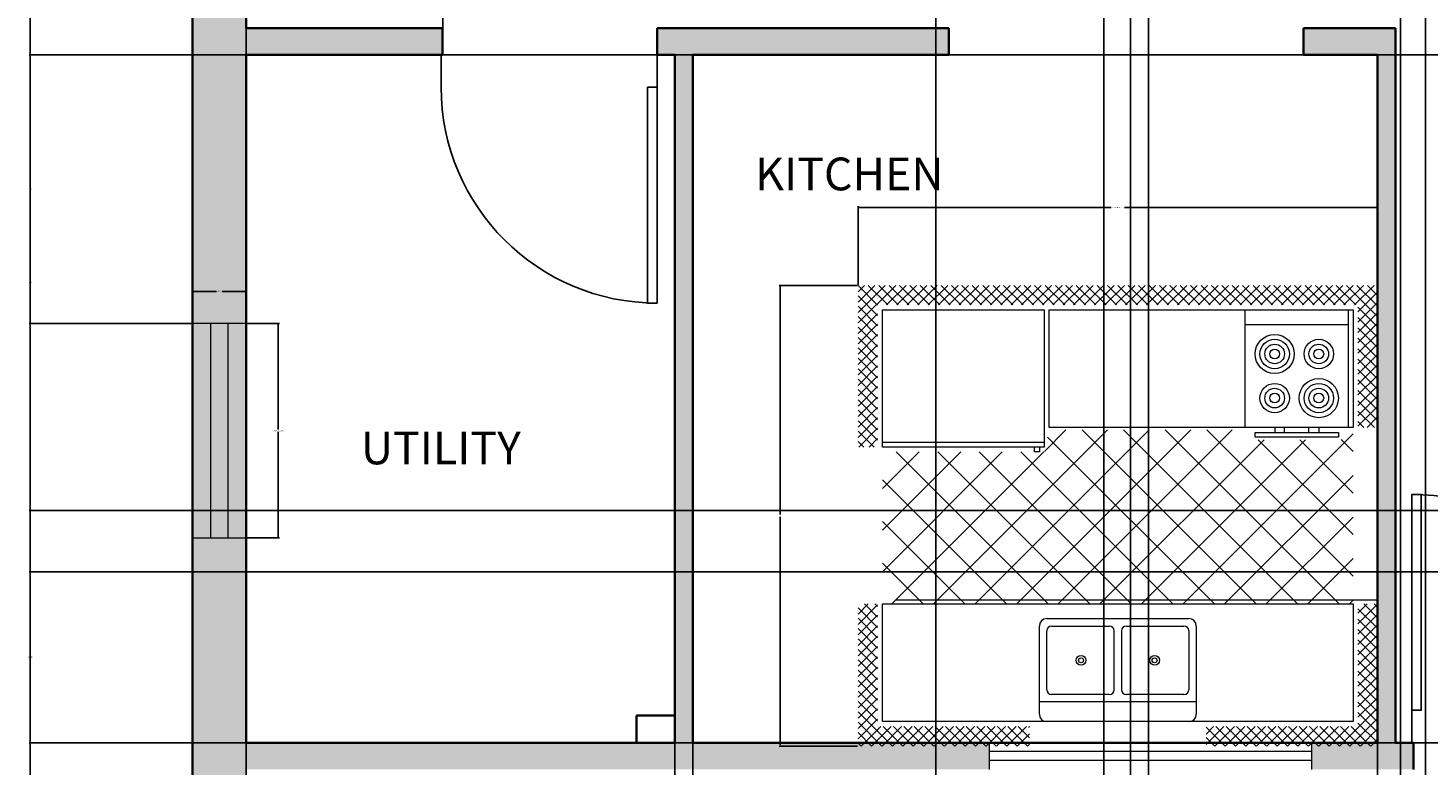
# Model space of a CAD drawing. Units: inches. Extents: x 1839 to 2285, y 722 to 1311.
# Tile 2 of 7: x 1870 to 2105, y 894 to 1018. Entities that reach past the tile are written whole.
import ezdxf

# ---------------------------------------------------------------- set-up
doc = ezdxf.new("R2010")
doc.units = ezdxf.units.IN
for name, color, linetype, lineweight in [('A-ANNO-DIMS', 2, 'Continuous', 18), ('A-AREA-IDEN', 7, 'Continuous', 18), ('A-DOOR', 3, 'Continuous', 25), ('A-FLOR-FIXT', 9, 'Continuous', 18), ('A-GLAZ', 4, 'Continuous', 18), ('A-GLAZ-PATT', 9, 'Continuous', 13), ('A-WALL', 7, 'Continuous', 35)]:
    doc.layers.add(name, color=color, linetype=linetype, lineweight=lineweight)
doc.layers.add('A-WALL-PATT', color=18, linetype='Continuous', lineweight=13, true_color=0x000000)
doc.styles.get("Standard").update_dxf_attribs({"font": 'arial.ttf'})
doc.dimstyles.get("Standard").update_dxf_attribs({"dimtxt": 0.18, "dimasz": 0.18, "dimexe": 0.18, "dimexo": 0.0625, "dimgap": 0.09, "dimtad": 0, "dimtih": 1, "dimtoh": 1, "dimdec": 4, "dimzin": 0, "dimdsep": 46, "dimtxsty": 'Standard', "dimcen": 0.09, "dimadec": 0, "dimazin": 0, "dimtfac": 1, "dimtdec": 4, "dimtofl": 0, "dimtmove": 0, "dimatfit": 3, "dimfxl": 1, "dimtolj": 1, "dimtzin": 0, "dimarcsym": 0})

# ---------------------------------------------------------------- blocks, each defined once
blk = doc.blocks.new('*U4')
for p, q in [((0, 0), (0, -6)), ((40, 0), (40, -6))]:
    blk.add_line(p, q)
blk.add_lwpolyline([(0, 0), (0, 40), (1.75, 40), (1.75, 0)], close=True)
blk.add_arc((0, 0), 40, 0, 90)
blk = doc.blocks.new('*U5')
for p, q in [((0, 0), (0, -6)), ((40, 0), (40, -6))]:
    blk.add_line(p, q)
blk.add_lwpolyline([(0, 0), (0, 40), (1.75, 40), (1.75, 0)], close=True)
blk.add_arc((0, 0), 40, 0, 90)
blk = doc.blocks.new('Kitchen Layout - 7 x 8 ft')
for p, q in [((-5, 81.32), (2.68, 89)), ((-5, 83.44), (0.56, 89)), ((-5, 85.56), (-1.56, 89)), ((-5, 87.68), (-3.68, 89)), ((-1, 84.97), (-5, 88.97)), ((1.09, 85), (-2.91, 89)), ((3.21, 85), (-0.79, 89)), ((0.81, 85), (4.81, 89)), ((5.34, 85), (1.34, 89)), ((2.93, 85), (6.93, 89)), ((7.46, 85), (3.46, 89)), ((5.05, 85), (9.05, 89)), ((9.58, 85), (5.58, 89)), ((7.17, 85), (11.17, 89)), ((11.7, 85), (7.7, 89)), ((9.29, 85), (13.29, 89)), ((13.82, 85), (9.82, 89)), ((11.41, 85), (15.41, 89)), ((15.94, 85), (11.94, 89)), ((13.53, 85), (17.53, 89)), ((18.06, 85), (14.06, 89)), ((15.65, 85), (19.65, 89)), ((20.18, 85), (16.18, 89)), ((17.78, 85), (21.78, 89)), ((22.31, 85), (18.31, 89)), ((19.9, 85), (23.9, 89)), ((24.43, 85), (20.43, 89)), ((22.02, 85), (26.02, 89)), ((26.55, 85), (22.55, 89)), ((24.14, 85), (28.14, 89)), ((28.67, 85), (24.67, 89)), ((26.26, 85), (30.26, 89)), ((30.79, 85), (26.79, 89)), ((28.38, 85), (32.38, 89)), ((32.91, 85), (28.91, 89)), ((30.5, 85), (34.5, 89)), ((35.03, 85), (31.03, 89)), ((32.63, 85), (36.63, 89)), ((37.16, 85), (33.16, 89)), ((34.75, 85), (38.75, 89)), ((39.28, 85), (35.28, 89)), ((36.87, 85), (40.87, 89)), ((41.4, 85), (37.4, 89)), ((38.99, 85), (42.99, 89)), ((43.52, 85), (39.52, 89)), ((41.11, 85), (45.11, 89)), ((45.64, 85), (41.64, 89)), ((43.23, 85), (47.23, 89)), ((47.76, 85), (43.76, 89)), ((45.35, 85), (49.35, 89)), ((49.88, 85), (45.88, 89)), ((47.47, 85), (51.47, 89)), ((52, 85), (48, 89)), ((49.6, 85), (53.6, 89)), ((54.13, 85), (50.13, 89)), ((51.72, 85), (55.72, 89)), ((56.25, 85), (52.25, 89)), ((53.84, 85), (57.84, 89)), ((58.37, 85), (54.37, 89)), ((55.96, 85), (59.96, 89)), ((60.49, 85), (56.49, 89)), ((58.08, 85), (62.08, 89)), ((62.61, 85), (58.61, 89)), ((60.2, 85), (64.2, 89)), ((64.73, 85), (60.73, 89)), ((62.32, 85), (66.32, 89)), ((66.85, 85), (62.85, 89)), ((64.45, 85), (68.45, 89)), ((68.97, 85), (64.97, 89)), ((66.57, 85), (70.57, 89)), ((71.1, 85), (67.1, 89)), ((68.69, 85), (72.69, 89)), ((73.22, 85), (69.22, 89)), ((70.81, 85), (74.81, 89)), ((75.34, 85), (71.34, 89)), ((72.93, 85), (76.93, 89)), ((77.46, 85), (73.46, 89)), ((75.05, 85), (79.05, 89)), ((79.58, 85), (75.58, 89)), ((77.17, 85), (81.17, 89)), ((81.7, 85), (77.7, 89)), ((79.29, 85), (83.29, 89)), ((83.82, 85), (79.82, 89)), ((81.42, 85), (85.42, 89)), ((85.95, 85), (81.95, 89)), ((83.54, 85), (87.54, 89)), ((88.07, 85), (84.07, 89)), ((85.66, 85), (89.66, 89)), ((90.19, 85), (86.19, 89)), ((87.78, 85), (91.78, 89)), ((92.31, 85), (88.31, 89)), ((89.9, 85), (93.9, 89)), ((94.43, 85), (90.43, 89)), ((92.02, 85), (96.02, 89)), ((96.55, 85), (92.55, 89)), ((94.14, 85), (98.14, 89)), ((101, 82.67), (94.67, 89)), ((96.27, 85), (100.27, 89)), ((101, 84.79), (96.79, 89)), ((101, 86.92), (98.92, 89)), ((-1, 82.85), (-5, 86.85)), ((97, 83.61), (101, 87.61)), ((-1, 80.73), (-5, 84.73)), ((-5, 79.19), (-1, 83.19)), ((34, 84), (96, 84)), ((34, 60), (34, 84)), ((96, 84), (96, 60)), ((97, 81.49), (101, 85.49)), ((101, 80.55), (97, 84.55)), ((97, 79.37), (101, 83.37)), ((-1, 78.61), (-5, 82.61)), ((-5, 77.07), (-1, 81.07)), ((-1, 76.49), (-5, 80.49)), ((74, 81), (95, 81)), ((101, 78.43), (97, 82.43)), ((97, 77.25), (101, 81.25)), ((101, 76.31), (97, 80.31)), ((-5, 74.95), (-1, 78.95)), ((-1, 74.36), (-5, 78.36)), ((97, 75.13), (101, 79.13)), ((101, 74.19), (97, 78.19)), ((-5, 72.83), (-1, 76.83)), ((-1, 72.24), (-5, 76.24)), ((-5, 70.71), (-1, 74.71)), ((97, 73.01), (101, 77.01)), ((101, 72.07), (97, 76.07)), ((97, 70.89), (101, 74.89)), ((-1, 70.12), (-5, 74.12)), ((-5, 68.59), (-1, 72.59)), ((-1, 68), (-5, 72)), ((101, 69.95), (97, 73.95)), ((97, 68.76), (101, 72.76)), ((101, 67.82), (97, 71.82)), ((-5, 66.47), (-1, 70.47)), ((-1, 65.88), (-5, 69.88)), ((97, 66.64), (101, 70.64)), ((101, 65.7), (97, 69.7)), ((-5, 64.35), (-1, 68.35)), ((-1, 63.76), (-5, 67.76)), ((-5, 62.22), (-1, 66.22)), ((97, 64.52), (101, 68.52)), ((101, 63.58), (97, 67.58)), ((97, 62.4), (101, 66.4)), ((-1, 61.64), (-5, 65.64)), ((-5, 60.1), (-1, 64.1)), ((-1, 59.52), (-5, 63.52)), ((101, 61.46), (97, 65.46)), ((97, 60.28), (101, 64.28)), ((100.34, 60), (97, 63.34)), ((-5, 57.98), (-1, 61.98)), ((-1, 57.39), (-5, 61.39)), ((96, 60), (34, 60)), ((80, 60), (80, 59)), ((82, 59), (82, 60)), ((87, 59), (87, 60)), ((89, 60), (89, 59)), ((98.22, 60), (97, 61.22)), ((98.84, 60), (101, 62.16)), ((100.96, 60), (101, 60.04)), ((-1.73, 56), (-5, 59.27)), ((-3.85, 56), (-5, 57.15)), ((-4.86, 56), (-1, 59.86)), ((-2.74, 56), (-1, 57.74)), ((10.4, 24), (45.9, 59.5)), ((18.88, 24), (54.38, 59.5)), ((27.37, 24), (62.87, 59.5)), ((33.03, 55.11), (37.41, 59.5)), ((67.71, 24), (33.68, 58.04)), ((35.85, 24), (71.35, 59.5)), ((76.2, 24), (40.7, 59.5)), ((44.34, 24), (77.84, 57.5)), ((84.68, 24), (49.18, 59.5)), ((52.82, 24), (86.32, 57.5)), ((93.17, 24), (57.67, 59.5)), ((61.31, 24), (96, 58.69)), ((96, 29.65), (66.15, 59.5)), ((96, 38.14), (76.64, 57.5)), ((96, 46.63), (85.13, 57.5)), ((96, 55.11), (93.57, 57.54)), ((0, 57), (33, 57)), ((0, 30.57), (24.43, 55)), ((0, 39.06), (15.94, 55)), ((0, 47.54), (7.46, 55)), ((1.91, 24), (32.91, 55)), ((33.77, 24), (2.77, 55)), ((42.26, 24), (11.26, 55)), ((50.74, 24), (19.74, 55)), ((59.23, 24), (28.23, 55)), ((31, 55), (31, 56)), ((32, 55), (31, 55)), ((32, 56), (32, 55)), ((25.29, 24), (0, 49.29)), ((69.79, 24), (96, 50.21)), ((16.8, 24), (0, 40.8)), ((78.28, 24), (96, 41.72)), ((8.32, 24), (0, 32.32)), ((86.76, 24), (96, 33.24)), ((-5, 21.92), (-2.92, 24)), ((-5, 19.8), (-1, 23.8)), ((-1, 19.21), (-5, 23.21)), ((-1, 21.33), (-3.67, 24)), ((-1, 23.45), (-1.55, 24)), ((0, 24), (96, 24)), ((0, 0), (0, 24)), ((95.25, 24), (96, 24.75)), ((96, 24), (96, 0)), ((97, 22.1), (98.9, 24)), ((97, 19.97), (101, 23.97)), ((101, 19.03), (97, 23.03)), ((101, 21.16), (98.16, 24)), ((101, 23.28), (100.28, 24)), ((-5, 17.68), (-1, 21.68)), ((-1, 17.09), (-5, 21.09)), ((97, 17.85), (101, 21.85)), ((101, 16.91), (97, 20.91)), ((-5, 15.55), (-1, 19.55)), ((-1, 14.97), (-5, 18.97)), ((-5, 13.43), (-1, 17.43)), ((47.25, 6.5), (47.25, 18.5)), ((48.75, 18.5), (48.75, 6.5)), ((97, 15.73), (101, 19.73)), ((101, 14.79), (97, 18.79)), ((97, 13.61), (101, 17.61)), ((-1, 12.85), (-5, 16.85)), ((-5, 11.31), (-1, 15.31)), ((-1, 10.73), (-5, 14.73)), ((101, 12.67), (97, 16.67)), ((97, 11.49), (101, 15.49)), ((101, 10.55), (97, 14.55)), ((-5, 9.19), (-1, 13.19)), ((-1, 8.6), (-5, 12.6)), ((97, 9.37), (101, 13.37)), ((101, 8.43), (97, 12.43)), ((-5, 7.07), (-1, 11.07)), ((-1, 6.48), (-5, 10.48)), ((-5, 4.95), (-1, 8.95)), ((97, 7.25), (101, 11.25)), ((101, 6.31), (97, 10.31)), ((97, 5.12), (101, 9.12)), ((-1, 4.36), (-5, 8.36)), ((-5, 2.83), (-1, 6.83)), ((-1, 2.24), (-5, 6.24)), ((101, 4.18), (97, 8.18)), ((97, 3), (101, 7)), ((101, 2.06), (97, 6.06)), ((-5, 0.71), (-1, 4.71)), ((-1, 0.12), (-5, 4.12)), ((64, 4), (32, 4)), ((97, 0.88), (101, 4.88)), ((101, -0.06), (97, 3.94)), ((-5, -1.42), (-1, 2.58)), ((2, -5), (-5, 2)), ((-5, -3.54), (-1, 0.46)), ((96, 0), (0, 0)), ((93.24, -5), (101, 2.76)), ((95.36, -5), (101, 0.64)), ((101, -2.18), (97, 1.82)), ((-0.12, -5), (-5, -0.12)), ((-2.25, -5), (-5, -2.25)), ((-4.34, -5), (-0.34, -1)), ((-2.22, -5), (1.78, -1)), ((-0.1, -5), (3.9, -1)), ((4.12, -5), (0.12, -1)), ((2.02, -5), (6.02, -1)), ((6.24, -5), (2.24, -1)), ((4.14, -5), (8.14, -1)), ((8.36, -5), (4.36, -1)), ((6.27, -5), (10.27, -1)), ((10.48, -5), (6.48, -1)), ((8.39, -5), (12.39, -1)), ((12.6, -5), (8.6, -1)), ((10.51, -5), (14.51, -1)), ((14.73, -5), (10.73, -1)), ((12.63, -5), (16.63, -1)), ((16.85, -5), (12.85, -1)), ((14.75, -5), (18.75, -1)), ((18.97, -5), (14.97, -1)), ((16.87, -5), (20.87, -1)), ((21.09, -5), (17.09, -1)), ((18.99, -5), (22.99, -1)), ((23.21, -5), (19.21, -1)), ((21.11, -5), (25.11, -1)), ((25.33, -5), (21.33, -1)), ((23.24, -5), (27.24, -1)), ((27.45, -5), (23.45, -1)), ((25.36, -5), (29.36, -1)), ((29.57, -5), (25.57, -1)), ((27.48, -5), (30, -2.48)), ((30, -3.3), (27.7, -1)), ((30, -1.18), (29.82, -1)), ((66, -2.54), (67.54, -1)), ((66, -4.66), (69.66, -1)), ((69.88, -5), (66, -1.12)), ((67.78, -5), (71.78, -1)), ((72, -5), (68, -1)), ((69.9, -5), (73.9, -1)), ((74.12, -5), (70.12, -1)), ((72.03, -5), (76.03, -1)), ((76.24, -5), (72.24, -1)), ((74.15, -5), (78.15, -1)), ((78.36, -5), (74.36, -1)), ((76.27, -5), (80.27, -1)), ((80.49, -5), (76.49, -1)), ((78.39, -5), (82.39, -1)), ((82.61, -5), (78.61, -1)), ((80.51, -5), (84.51, -1)), ((84.73, -5), (80.73, -1)), ((82.63, -5), (86.63, -1)), ((86.85, -5), (82.85, -1)), ((84.75, -5), (88.75, -1)), ((88.97, -5), (84.97, -1)), ((86.88, -5), (90.88, -1)), ((91.09, -5), (87.09, -1)), ((89, -5), (93, -1)), ((93.21, -5), (89.21, -1)), ((91.12, -5), (95.12, -1)), ((95.34, -5), (91.34, -1)), ((97.46, -5), (93.46, -1)), ((99.58, -5), (95.58, -1)), ((101, -4.3), (97, -0.3)), ((97.48, -5), (101, -1.48)), ((-4.37, -5), (-5, -4.37)), ((29.6, -5), (30, -4.6)), ((67.76, -5), (66, -3.24)), ((99.6, -5), (101, -3.6))]:
    blk.add_line(p, q)
for points in [[(0, 56), (0, 84), (33, 84), (33, 56)], [(74, 60), (74, 84), (95, 84), (95, 60)], [(76, 58), (76, 59), (93, 59), (93, 58)]]:
    blk.add_lwpolyline(points, close=True)
for points in [[(33.5, 21), (62.5, 21)], [(32, 1.5), (32, 19.5)], [(33.5, 6.5), (33.5, 18.5)], [(34.5, 19.5), (46.25, 19.5)], [(49.75, 19.5), (61.5, 19.5)], [(62.5, 18.5), (62.5, 6.5)], [(64, 19.5), (64, 1.5)], [(46.25, 5.5), (34.5, 5.5)], [(61.5, 5.5), (49.75, 5.5)], [(62.5, 0), (33.5, 0)]]:
    blk.add_lwpolyline(points)
for centre, radius in [((80, 75), 4), ((80, 75), 3), ((89, 75), 3), ((80, 75), 2), ((80, 75), 1), ((89, 75), 2), ((89, 75), 1), ((80, 66), 3), ((89, 66), 4), ((89, 66), 3), ((80, 66), 2), ((80, 66), 1), ((89, 66), 2), ((89, 66), 1), ((40.5, 12.5), 1), ((40.5, 12.5), 0.5), ((55.5, 12.5), 1), ((55.5, 12.5), 0.5)]:
    blk.add_circle(centre, radius)
for centre, radius, start, end in [((33.5, 19.5), 1.5, 90, 180), ((62.5, 19.5), 1.5, 0, 90), ((34.5, 18.5), 1, 90, 180), ((46.25, 18.5), 1, 0, 90), ((49.75, 18.5), 1, 90, 180), ((61.5, 18.5), 1, 0, 90), ((34.5, 6.5), 1, 180, 270), ((46.25, 6.5), 1, 270, 0), ((49.75, 6.5), 1, 180, 270), ((61.5, 6.5), 1, 270, 0), ((33.5, 1.5), 1.5, 180, 270), ((62.5, 1.5), 1.5, 270, 0)]:
    blk.add_arc(centre, radius, start, end)
blk = doc.blocks.new('WIN-36x9')
for p, q in [((0, 9), (0, 0)), ((36, 9), (0, 9)), ((36, 0), (36, 9)), ((36, 6), (0, 6)), ((0, 3), (36, 3)), ((0, 0), (36, 0))]:
    blk.add_line(p, q)
blk = doc.blocks.new('*D19')
at = {"layer": 'A-ANNO-DIMS', "color": 0, "lineweight": -2, "transparency": 16777216}
for p, q in [((1906.74, 968.21), (1912.26, 968.21)), ((1912.08, 968.03), (1912.08, 950.39)), ((1912.08, 932.39), (1912.08, 950.03)), ((1906.74, 932.21), (1912.26, 932.21))]:
    blk.add_line(p, q, dxfattribs=at)
at = {"layer": 'A-ANNO-DIMS', "color": 0, "transparency": 16777216}
for points in [[(1912.05, 968.03), (1912.11, 968.03), (1912.08, 968.21)], [(1912.05, 932.39), (1912.11, 932.39), (1912.08, 932.21)]]:
    blk.add_solid(points, dxfattribs=at)
at = {"layer": 'Defpoints', "color": 0, "transparency": 16777216}
for p in [(1906.68, 968.21), (1906.68, 932.21), (1912.08, 932.21)]:
    blk.add_point(p, dxfattribs=at)
at = {"layer": 'A-ANNO-DIMS', "color": 0, "transparency": 16777216, "insert": (1912.08, 950.21), "char_height": 0.18, "attachment_point": 5}
blk.add_mtext('\\A1;WINDOW 36 TYP.', dxfattribs=at)
blk = doc.blocks.new('*D20')
at = {"layer": 'A-ANNO-DIMS', "color": 0, "lineweight": -2, "transparency": 16777216}
for p, q in [((1897.68, 968.27), (1897.68, 973.79)), ((1897.86, 973.61), (1901.72, 973.61)), ((1906.5, 973.61), (1902.64, 973.61)), ((1906.68, 968.27), (1906.68, 973.79))]:
    blk.add_line(p, q, dxfattribs=at)
at = {"layer": 'A-ANNO-DIMS', "color": 0, "transparency": 16777216}
for points in [[(1897.86, 973.64), (1897.86, 973.58), (1897.68, 973.61)], [(1906.5, 973.64), (1906.5, 973.58), (1906.68, 973.61)]]:
    blk.add_solid(points, dxfattribs=at)
at = {"layer": 'Defpoints', "color": 0, "transparency": 16777216}
for p in [(1906.68, 973.61), (1897.68, 968.21), (1906.68, 968.21)]:
    blk.add_point(p, dxfattribs=at)
at = {"layer": 'A-ANNO-DIMS', "color": 0, "transparency": 16777216, "insert": (1902.18, 973.61), "char_height": 0.18, "attachment_point": 5}
blk.add_mtext('\\A1;9 TYP.', dxfattribs=at)
blk = doc.blocks.new('*D35')
at = {"layer": 'A-ANNO-DIMS', "color": 0, "lineweight": -2, "transparency": 16777216}
for p, q in [((2009.42, 974.68), (2009.42, 987.89)), ((2009.6, 987.71), (2051.91, 987.71)), ((2096.48, 987.71), (2054.17, 987.71)), ((2096.66, 974.68), (2096.66, 987.89))]:
    blk.add_line(p, q, dxfattribs=at)
at = {"layer": 'A-ANNO-DIMS', "color": 0, "transparency": 16777216}
for points in [[(2009.6, 987.74), (2009.6, 987.68), (2009.42, 987.71)], [(2096.48, 987.74), (2096.48, 987.68), (2096.66, 987.71)]]:
    blk.add_solid(points, dxfattribs=at)
at = {"layer": 'Defpoints', "color": 0, "transparency": 16777216}
for p in [(2096.66, 987.71), (2009.42, 974.62), (2096.66, 974.62)]:
    blk.add_point(p, dxfattribs=at)
at = {"layer": 'A-ANNO-DIMS', "color": 0, "transparency": 16777216, "insert": (2053.04, 987.71), "char_height": 0.18, "attachment_point": 5}
blk.add_mtext('\\A1;KITCHEN UNIT 87', dxfattribs=at)
blk = doc.blocks.new('*D36')
at = {"layer": 'A-ANNO-DIMS', "color": 0, "lineweight": -2, "transparency": 16777216}
for p, q in [((2009.36, 974.62), (1996.16, 974.62)), ((1996.34, 974.44), (1996.34, 936.12)), ((1996.34, 897.44), (1996.34, 935.76)), ((2009.36, 897.26), (1996.16, 897.26))]:
    blk.add_line(p, q, dxfattribs=at)
at = {"layer": 'A-ANNO-DIMS', "color": 0, "transparency": 16777216}
for points in [[(1996.31, 974.44), (1996.37, 974.44), (1996.34, 974.62)], [(1996.31, 897.44), (1996.37, 897.44), (1996.34, 897.26)]]:
    blk.add_solid(points, dxfattribs=at)
at = {"layer": 'Defpoints', "color": 0, "transparency": 16777216}
for p in [(1996.34, 974.62), (2009.42, 974.62), (2009.42, 897.26)]:
    blk.add_point(p, dxfattribs=at)
at = {"layer": 'A-ANNO-DIMS', "color": 0, "transparency": 16777216, "insert": (1996.34, 935.94), "char_height": 0.18, "attachment_point": 5}
blk.add_mtext('\\A1;77', dxfattribs=at)
blk = doc.blocks.new('*D42')
at = {"layer": 'A-ANNO-DIMS', "color": 0, "lineweight": -2, "transparency": 16777216}
for p, q in [((1897.61, 1283.33), (1870.25, 1283.33)), ((1870.43, 1283.15), (1870.43, 1043.51)), ((1870.43, 803.51), (1870.43, 1043.15)), ((1897.61, 803.33), (1870.25, 803.33))]:
    blk.add_line(p, q, dxfattribs=at)
at = {"layer": 'A-ANNO-DIMS', "color": 0, "transparency": 16777216}
for points in [[(1870.4, 1283.15), (1870.46, 1283.15), (1870.43, 1283.33)], [(1870.4, 803.51), (1870.46, 803.51), (1870.43, 803.33)]]:
    blk.add_solid(points, dxfattribs=at)
at = {"layer": 'Defpoints', "color": 0, "transparency": 16777216}
for p in [(1870.43, 1283.33), (1897.68, 1283.33), (1897.68, 803.33)]:
    blk.add_point(p, dxfattribs=at)
at = {"layer": 'A-ANNO-DIMS', "color": 0, "transparency": 16777216, "insert": (1870.43, 1043.33), "char_height": 0.18, "attachment_point": 5}
blk.add_mtext('\\A1;480', dxfattribs=at)
blk = doc.blocks.new('*D43')
at = {"layer": 'A-ANNO-DIMS', "color": 0, "lineweight": -2, "transparency": 16777216}
for p, q in [((2050.68, 1145.27), (2050.68, 722.34)), ((1906.68, 1142.27), (1906.68, 722.34)), ((1906.86, 722.52), (1978.4, 722.52)), ((2050.5, 722.52), (1978.96, 722.52))]:
    blk.add_line(p, q, dxfattribs=at)
at = {"layer": 'A-ANNO-DIMS', "color": 0, "transparency": 16777216}
for points in [[(1906.86, 722.55), (1906.86, 722.49), (1906.68, 722.52)], [(2050.5, 722.55), (2050.5, 722.49), (2050.68, 722.52)]]:
    blk.add_solid(points, dxfattribs=at)
at = {"layer": 'Defpoints', "color": 0, "transparency": 16777216}
for p in [(2050.68, 1145.33), (1906.68, 1142.33), (2050.68, 722.52)]:
    blk.add_point(p, dxfattribs=at)
at = {"layer": 'A-ANNO-DIMS', "color": 0, "transparency": 16777216, "insert": (1978.68, 722.52), "char_height": 0.18, "attachment_point": 5}
blk.add_mtext('\\A1;144', dxfattribs=at)
blk = doc.blocks.new('*D44')
at = {"layer": 'A-ANNO-DIMS', "color": 0, "lineweight": -2, "transparency": 16777216}
for p, q in [((2055.18, 1137.77), (2055.18, 722.34)), ((2104.68, 1137.77), (2104.68, 722.34)), ((2055.36, 722.52), (2079.6, 722.52)), ((2104.5, 722.52), (2080.26, 722.52))]:
    blk.add_line(p, q, dxfattribs=at)
at = {"layer": 'A-ANNO-DIMS', "color": 0, "transparency": 16777216}
for points in [[(2055.36, 722.55), (2055.36, 722.49), (2055.18, 722.52)], [(2104.5, 722.55), (2104.5, 722.49), (2104.68, 722.52)]]:
    blk.add_solid(points, dxfattribs=at)
at = {"layer": 'Defpoints', "color": 0, "transparency": 16777216}
for p in [(2055.18, 1137.83), (2104.68, 1137.83), (2104.68, 722.52)]:
    blk.add_point(p, dxfattribs=at)
at = {"layer": 'A-ANNO-DIMS', "color": 0, "transparency": 16777216, "insert": (2079.93, 722.52), "char_height": 0.18, "attachment_point": 5}
blk.add_mtext('\\A1;49.5', dxfattribs=at)
blk = doc.blocks.new('*D51')
at = {"layer": 'A-ANNO-DIMS', "color": 0, "lineweight": -2, "transparency": 16777216}
for p, q in [((1906.68, 897.77), (1906.68, 722.34)), ((1978.68, 897.77), (1978.68, 722.34)), ((1906.86, 722.52), (1942.46, 722.52)), ((1978.5, 722.52), (1942.89, 722.52))]:
    blk.add_line(p, q, dxfattribs=at)
at = {"layer": 'A-ANNO-DIMS', "color": 0, "transparency": 16777216}
for points in [[(1906.86, 722.55), (1906.86, 722.49), (1906.68, 722.52)], [(1978.5, 722.55), (1978.5, 722.49), (1978.68, 722.52)]]:
    blk.add_solid(points, dxfattribs=at)
at = {"layer": 'Defpoints', "color": 0, "transparency": 16777216}
for p in [(1906.68, 897.83), (1978.68, 897.83), (1978.68, 722.52)]:
    blk.add_point(p, dxfattribs=at)
at = {"layer": 'A-ANNO-DIMS', "color": 0, "transparency": 16777216, "insert": (1942.68, 722.52), "char_height": 0.18, "attachment_point": 5}
blk.add_mtext('\\A1;72', dxfattribs=at)
blk = doc.blocks.new('*D52')
at = {"layer": 'A-ANNO-DIMS', "color": 0, "lineweight": -2, "transparency": 16777216}
for p, q in [((1981.68, 1013.27), (1981.68, 722.34)), ((2096.66, 1013.27), (2096.66, 722.34)), ((1981.86, 722.52), (2038.72, 722.52)), ((2096.48, 722.52), (2039.63, 722.52))]:
    blk.add_line(p, q, dxfattribs=at)
at = {"layer": 'A-ANNO-DIMS', "color": 0, "transparency": 16777216}
for points in [[(1981.86, 722.55), (1981.86, 722.49), (1981.68, 722.52)], [(2096.48, 722.55), (2096.48, 722.49), (2096.66, 722.52)]]:
    blk.add_solid(points, dxfattribs=at)
at = {"layer": 'Defpoints', "color": 0, "transparency": 16777216}
for p in [(1981.68, 1013.33), (2096.66, 1013.33), (2096.66, 722.52)]:
    blk.add_point(p, dxfattribs=at)
at = {"layer": 'A-ANNO-DIMS', "color": 0, "transparency": 16777216, "insert": (2039.17, 722.52), "char_height": 0.18, "attachment_point": 5}
blk.add_mtext('\\A1;114.99', dxfattribs=at)
blk = doc.blocks.new('*D55')
at = {"layer": 'A-ANNO-DIMS', "color": 0, "lineweight": -2, "transparency": 16777216}
for p, q in [((2022.5, 812.39), (2022.5, 1310.76)), ((2022.68, 1310.58), (2061.29, 1310.58)), ((2100.32, 1310.58), (2061.72, 1310.58)), ((2100.5, 812.39), (2100.5, 1310.76))]:
    blk.add_line(p, q, dxfattribs=at)
at = {"layer": 'A-ANNO-DIMS', "color": 0, "transparency": 16777216}
for points in [[(2022.68, 1310.61), (2022.68, 1310.55), (2022.5, 1310.58)], [(2100.32, 1310.61), (2100.32, 1310.55), (2100.5, 1310.58)]]:
    blk.add_solid(points, dxfattribs=at)
at = {"layer": 'Defpoints', "color": 0, "transparency": 16777216}
for p in [(2100.5, 1310.58), (2022.5, 812.33), (2100.5, 812.33)]:
    blk.add_point(p, dxfattribs=at)
at = {"layer": 'A-ANNO-DIMS', "color": 0, "transparency": 16777216, "insert": (2061.5, 1310.58), "char_height": 0.18, "attachment_point": 5}
blk.add_mtext('\\A1;78', dxfattribs=at)
blk = doc.blocks.new('*D63')
at = {"layer": 'A-ANNO-DIMS', "color": 0, "lineweight": -2, "transparency": 16777216}
for p, q in [((1906.61, 1013.33), (1870.25, 1013.33)), ((1870.43, 1013.15), (1870.43, 990.95)), ((1870.43, 968.39), (1870.43, 990.59)), ((1897.61, 968.21), (1870.25, 968.21))]:
    blk.add_line(p, q, dxfattribs=at)
at = {"layer": 'A-ANNO-DIMS', "color": 0, "transparency": 16777216}
for points in [[(1870.4, 1013.15), (1870.46, 1013.15), (1870.43, 1013.33)], [(1870.4, 968.39), (1870.46, 968.39), (1870.43, 968.21)]]:
    blk.add_solid(points, dxfattribs=at)
at = {"layer": 'Defpoints', "color": 0, "transparency": 16777216}
for p in [(1870.43, 1013.33), (1906.68, 1013.33), (1897.68, 968.21)]:
    blk.add_point(p, dxfattribs=at)
at = {"layer": 'A-ANNO-DIMS', "color": 0, "transparency": 16777216, "insert": (1870.43, 990.77), "char_height": 0.18, "attachment_point": 5}
blk.add_mtext('\\A1;45.12', dxfattribs=at)
blk = doc.blocks.new('*D64')
at = {"layer": 'A-ANNO-DIMS', "color": 0, "lineweight": -2, "transparency": 16777216}
for p, q in [((2248.61, 926.49), (1870.25, 926.49)), ((1870.43, 926.31), (1870.43, 912.34)), ((1870.43, 898.01), (1870.43, 911.98)), ((2248.61, 897.83), (1870.25, 897.83))]:
    blk.add_line(p, q, dxfattribs=at)
at = {"layer": 'A-ANNO-DIMS', "color": 0, "transparency": 16777216}
for points in [[(1870.4, 926.31), (1870.46, 926.31), (1870.43, 926.49)], [(1870.4, 898.01), (1870.46, 898.01), (1870.43, 897.83)]]:
    blk.add_solid(points, dxfattribs=at)
at = {"layer": 'Defpoints', "color": 0, "transparency": 16777216}
for p in [(1870.43, 926.49), (2248.68, 926.49), (2248.68, 897.83)]:
    blk.add_point(p, dxfattribs=at)
at = {"layer": 'A-ANNO-DIMS', "color": 0, "transparency": 16777216, "insert": (1870.43, 912.16), "char_height": 0.18, "attachment_point": 5}
blk.add_mtext('\\A1;28.655', dxfattribs=at)
blk = doc.blocks.new('*D71')
at = {"layer": 'A-ANNO-DIMS', "color": 0, "lineweight": -2, "transparency": 16777216}
for p, q in [((1978.68, 897.77), (1978.68, 722.34)), ((1981.68, 897.77), (1981.68, 722.34)), ((1978.86, 722.52), (1980.03, 722.52)), ((1981.5, 722.52), (1980.33, 722.52))]:
    blk.add_line(p, q, dxfattribs=at)
at = {"layer": 'A-ANNO-DIMS', "color": 0, "transparency": 16777216}
for points in [[(1978.86, 722.55), (1978.86, 722.49), (1978.68, 722.52)], [(1981.5, 722.55), (1981.5, 722.49), (1981.68, 722.52)]]:
    blk.add_solid(points, dxfattribs=at)
at = {"layer": 'Defpoints', "color": 0, "transparency": 16777216}
for p in [(1978.68, 897.83), (1981.68, 897.83), (1981.68, 722.52)]:
    blk.add_point(p, dxfattribs=at)
at = {"layer": 'A-ANNO-DIMS', "color": 0, "transparency": 16777216, "insert": (1980.18, 722.52), "char_height": 0.18, "attachment_point": 5}
blk.add_mtext('\\A1;3', dxfattribs=at)
blk = doc.blocks.new('*D81')
at = {"layer": 'A-ANNO-DIMS', "color": 0, "lineweight": -2, "transparency": 16777216}
for p, q in [((1906.68, 1013.39), (1906.68, 1310.76)), ((1906.86, 1310.58), (1922.96, 1310.58)), ((1939.5, 1310.58), (1923.4, 1310.58)), ((1939.68, 1013.39), (1939.68, 1310.76))]:
    blk.add_line(p, q, dxfattribs=at)
at = {"layer": 'A-ANNO-DIMS', "color": 0, "transparency": 16777216}
for points in [[(1906.86, 1310.61), (1906.86, 1310.55), (1906.68, 1310.58)], [(1939.5, 1310.61), (1939.5, 1310.55), (1939.68, 1310.58)]]:
    blk.add_solid(points, dxfattribs=at)
at = {"layer": 'Defpoints', "color": 0, "transparency": 16777216}
for p in [(1939.68, 1310.58), (1906.68, 1013.33), (1939.68, 1013.33)]:
    blk.add_point(p, dxfattribs=at)
at = {"layer": 'A-ANNO-DIMS', "color": 0, "transparency": 16777216, "insert": (1923.18, 1310.58), "char_height": 0.18, "attachment_point": 5}
blk.add_mtext('\\A1;33', dxfattribs=at)
blk = doc.blocks.new('*D82')
at = {"layer": 'A-ANNO-DIMS', "color": 0, "lineweight": -2, "transparency": 16777216}
for p, q in [((2164.61, 1013.33), (1870.25, 1013.33)), ((1870.43, 1013.15), (1870.43, 975.26)), ((1870.43, 937.01), (1870.43, 974.9)), ((2164.61, 936.83), (1870.25, 936.83))]:
    blk.add_line(p, q, dxfattribs=at)
at = {"layer": 'A-ANNO-DIMS', "color": 0, "transparency": 16777216}
for points in [[(1870.4, 1013.15), (1870.46, 1013.15), (1870.43, 1013.33)], [(1870.4, 937.01), (1870.46, 937.01), (1870.43, 936.83)]]:
    blk.add_solid(points, dxfattribs=at)
at = {"layer": 'Defpoints', "color": 0, "transparency": 16777216}
for p in [(1870.43, 1013.33), (2164.68, 1013.33), (2164.68, 936.83)]:
    blk.add_point(p, dxfattribs=at)
at = {"layer": 'A-ANNO-DIMS', "color": 0, "transparency": 16777216, "insert": (1870.43, 975.08), "char_height": 0.18, "attachment_point": 5}
blk.add_mtext('\\A1;76.5', dxfattribs=at)
blk = doc.blocks.new('*D84')
at = {"layer": 'A-ANNO-DIMS', "color": 0, "lineweight": -2, "transparency": 16777216}
for p, q in [((2055.18, 1218.77), (2055.18, 722.34)), ((2058.18, 1218.77), (2058.18, 722.34)), ((2055.36, 722.52), (2056.53, 722.52)), ((2058, 722.52), (2056.83, 722.52))]:
    blk.add_line(p, q, dxfattribs=at)
at = {"layer": 'A-ANNO-DIMS', "color": 0, "transparency": 16777216}
for points in [[(2055.36, 722.55), (2055.36, 722.49), (2055.18, 722.52)], [(2058, 722.55), (2058, 722.49), (2058.18, 722.52)]]:
    blk.add_solid(points, dxfattribs=at)
at = {"layer": 'Defpoints', "color": 0, "transparency": 16777216}
for p in [(2055.18, 1218.83), (2058.18, 1218.83), (2058.18, 722.52)]:
    blk.add_point(p, dxfattribs=at)
at = {"layer": 'A-ANNO-DIMS', "color": 0, "transparency": 16777216, "insert": (2056.68, 722.52), "char_height": 0.18, "attachment_point": 5}
blk.add_mtext('\\A1;3', dxfattribs=at)

msp = doc.modelspace()

# ---------------------------------------------------------------- hatches: boundary and pattern name
at = {"layer": 'A-GLAZ-PATT'}
h = msp.add_hatch(color=256, dxfattribs=at)
h.dxf.hatch_style = 1
h.set_gradient(color1=(0, 0, 255), color2=(255, 255, 0), name='INVCYLINDER')
h.paths.add_polyline_path([(1900.6771, 968.2107), (1897.6771, 968.2107), (1897.6771, 932.2107), (1900.6771, 932.2107)])
h.paths.add_polyline_path([(1903.6771, 968.2107), (1900.6771, 968.2107), (1900.6771, 932.2107), (1903.6771, 932.2107)])
h.paths.add_polyline_path([(1906.6771, 968.2107), (1903.6771, 968.2107), (1903.6771, 932.2107), (1906.6771, 932.2107)])
at = {"layer": 'A-WALL-PATT'}
h = msp.add_hatch(color=256, dxfattribs=at)
h.dxf.hatch_style = 1
h.paths.add_polyline_path([(1906.6771, 1274.3314), (1942.6771, 1274.3314), (1942.6771, 1283.3314), (1897.6771, 1283.3314), (1897.6771, 968.2107), (1906.6771, 968.2107), (1906.6771, 1013.3314), (1939.6771, 1013.3314), (1939.6771, 1017.8314), (1906.6771, 1017.8314), (1906.6771, 1137.8314), (2050.6771, 1137.8314), (2050.6771, 1142.3314), (1906.6771, 1142.3314)])
h.paths.add_polyline_path([(2064.0508, 1283.3314), (1978.6771, 1283.3314), (1978.6771, 1274.3314), (2050.6771, 1274.3314), (2050.6771, 1184.3314), (2055.1771, 1184.3314), (2055.1771, 1214.3314), (2058.1771, 1214.3314), (2058.1771, 1218.8314), (2055.1771, 1218.8314), (2055.1771, 1274.3314), (2064.0508, 1274.3314)])
h.paths.add_polyline_path([(2182.6416, 1283.3314), (2088.0508, 1283.3314), (2088.0508, 1274.3314), (2104.6771, 1274.3314), (2104.6771, 1218.8314), (2094.1771, 1218.8314), (2094.1771, 1214.3314), (2104.6771, 1214.3314), (2104.6771, 1184.3314), (2109.1771, 1184.3314), (2109.1771, 1274.3314), (2182.6416, 1274.3314)])
h.paths.add_polyline_path([(2257.6771, 1283.3314), (2218.6416, 1283.3314), (2218.6416, 1274.3314), (2248.6771, 1274.3314), (2248.6771, 1142.3314), (2186.4004, 1142.3314), (2109.1771, 1142.3314), (2109.1771, 1137.8314), (2248.6771, 1137.8314), (2248.6771, 1094.9086), (2257.6771, 1094.9086)])
h.paths.add_polyline_path([(2257.6771, 1058.9086), (2248.6771, 1058.9086), (2248.6771, 1017.8314), (2160.1771, 1017.8314), (2160.1771, 939.8314), (2164.6771, 939.8314), (2164.6771, 1013.3314), (2248.6771, 1013.3314), (2248.6771, 977.3314), (2248.6771, 950.4862), (2257.6771, 950.4862)])
h.paths.add_polyline_path([(2257.6771, 893.3314), (2248.6771, 893.3314), (2248.6771, 850.1143), (2190.4862, 850.1143), (2190.4862, 845.6143), (2248.6771, 845.6143), (2248.6771, 812.3314), (2100.5038, 812.3314), (2100.5038, 803.3314), (2257.6771, 803.3314)])
h.paths.add_polyline_path([(2257.6771, 926.4862), (2248.6771, 926.4862), (2248.6771, 897.8314), (2141.6642, 897.8314), (2141.6642, 893.3314), (2145.5038, 893.3314), (2145.5038, 812.3314), (2147.5038, 812.3314), (2147.5038, 845.6143), (2153.9854, 845.6143), (2153.9854, 850.1143), (2147.5038, 850.1143), (2147.5038, 893.3314), (2248.6771, 893.3314), (2257.6771, 893.3314)])
h.paths.add_polyline_path([(1906.6771, 893.3314), (1897.6771, 893.3314), (1897.6771, 803.3314), (2022.5038, 803.3314), (2022.5038, 812.3314), (1906.6771, 812.3314)])
h.paths.add_polyline_path([(2031.4676, 897.8314), (1981.6771, 897.8314), (1981.6771, 1013.3314), (2024.6642, 1013.3314), (2024.6642, 1017.8314), (1975.6771, 1017.8314), (1975.6771, 1013.3314), (1978.6771, 1013.3314), (1978.6771, 897.8314), (1906.6771, 897.8314), (1906.6771, 932.2107), (1897.6771, 932.2107), (1897.6771, 893.3314), (1906.6771, 893.3314), (2031.4676, 893.3314)])
h.paths.add_polyline_path([(2099.6642, 1017.8314), (2096.6642, 1017.8314), (2084.1956, 1017.8314), (2084.1956, 1013.3314), (2096.6642, 1013.3314), (2096.6642, 897.8314), (2085.6129, 897.8314), (2085.6129, 893.3314), (2102.6642, 893.3314), (2102.6642, 897.8314), (2099.6642, 897.8314)])

# ---------------------------------------------------------------- linework, layer by layer
at = {"layer": 'A-FLOR-FIXT'}
msp.add_line((2015.8192, 921.8314), (2096.6642, 921.8314), dxfattribs=at)
at = {"layer": 'A-GLAZ'}
for p, q in [((2085.6129, 897.8314), (2031.4676, 897.8314)), ((2031.4676, 897.8314), (2031.4676, 893.3314)), ((2085.6129, 896.3314), (2031.4676, 896.3314)), ((2085.6129, 893.3314), (2085.6129, 897.8314)), ((2085.6129, 894.8314), (2031.4676, 894.8314))]:
    msp.add_line(p, q, dxfattribs=at)
at = {"layer": 'A-WALL'}
for p, q in [((1906.6771, 1017.8314), (1906.6771, 1137.8314)), ((1906.6771, 1017.8314), (1939.6771, 1017.8314)), ((1939.6771, 1013.3314), (1939.6771, 1017.8314)), ((1975.6771, 1013.3314), (1975.6771, 1017.8314)), ((1975.6771, 1017.8314), (2024.6642, 1017.8314)), ((2024.6642, 1013.3314), (2024.6642, 1017.8314)), ((2084.1956, 1013.3314), (2084.1956, 1017.8314)), ((2084.1956, 1017.8314), (2096.6642, 1017.8314)), ((2096.6642, 1017.8314), (2099.6642, 1017.8314)), ((2099.6642, 897.8314), (2099.6642, 1017.8314)), ((1906.6771, 1013.3314), (1939.6771, 1013.3314)), ((1906.6771, 897.8314), (1906.6771, 1013.3314)), ((1975.6771, 1013.3314), (1978.6771, 1013.3314)), ((1978.6771, 897.8314), (1978.6771, 1013.3314)), ((1981.6771, 897.8314), (1981.6771, 1013.3314)), ((1981.6771, 1013.3314), (2024.6642, 1013.3314)), ((2084.1956, 1013.3314), (2096.6642, 1013.3314)), ((2096.6642, 897.8314), (2096.6642, 1013.3314)), ((1972.2025, 897.8314), (1972.2025, 902.3685)), ((1972.2025, 902.3685), (1978.6771, 902.3685)), ((1906.6771, 897.8314), (1978.6771, 897.8314)), ((1981.6771, 897.8314), (2096.6642, 897.8314)), ((2099.6642, 897.8314), (2102.6642, 897.8314)), ((2102.6642, 893.3314), (2102.6642, 897.8314))]:
    msp.add_line(p, q, dxfattribs=at)
msp.add_lwpolyline([(2022.5038, 803.3314), (1897.6771, 803.3314), (1897.6771, 1283.3314), (2257.6771, 1283.3314), (2257.6771, 803.3314), (2100.5038, 803.3314)], dxfattribs=at)

# ---------------------------------------------------------------- block references
at = {"layer": 'A-DOOR', "xscale": 0.9062393225401889, "yscale": 0.9062393225401889, "zscale": 0.9062393225401889, "rotation": 180}
msp.add_blockref('*U4', (1975.6771, 1007.894), dxfattribs=at)
at = {"layer": 'A-DOOR', "xscale": 0.9062393225401889, "yscale": 0.9062393225401889, "zscale": 0.9062393225401889}
msp.add_blockref('*U5', (2102.4146, 903.2689), dxfattribs=at)
at = {"layer": 'A-FLOR-FIXT', "xscale": 0.8230300493925694, "yscale": 0.8230300493925694, "zscale": 0.8230300493925694}
msp.add_blockref('Kitchen Layout - 7 x 8 ft', (2013.5382, 901.371), dxfattribs=at)
at = {"layer": 'A-GLAZ', "rotation": 270.0000000000007}
msp.add_blockref('WIN-36x9', (1897.6767, 968.2103), dxfattribs=at)

# ---------------------------------------------------------------- texts
at = {"layer": 'A-AREA-IDEN'}
for s, p in [('KITCHEN ', (1992.1458, 990.5751)), ('UTILITY ', (1925.9365, 944.5691))]:
    msp.add_text(s, height=5.50379, dxfattribs=at).set_placement(p)

# ---------------------------------------------------------------- dimensions: what is measured, and where the dimension line sits
at = {"layer": 'A-ANNO-DIMS'}
for base, p1, p2, override, picture, middle in [((1939.6771, 1310.5814), (1906.6771, 1013.3314), (1939.6771, 1013.3314), {"dimdec": 0, "dimlfac": 1, "dimrnd": 0, "dimzin": 0, "dimdsep": 46, "dimlunit": 2}, '*D81', (1923.1771, 1310.5814)), ((2100.5038, 1310.5814), (2022.5038, 812.3314), (2100.5038, 812.3314), {"dimdec": 0, "dimlfac": 1, "dimrnd": 0, "dimzin": 0, "dimdsep": 46, "dimlunit": 2}, '*D55', (2061.5038, 1310.5814)), ((2058.1771, 722.516), (2055.1771, 1218.8314), (2058.1771, 1218.8314), {"dimdec": 0, "dimlfac": 1, "dimrnd": 0, "dimzin": 0, "dimdsep": 46, "dimlunit": 2}, '*D84', (2056.6771, 722.516)), ((2050.6771, 722.516), (1906.6771, 1142.3314), (2050.6771, 1145.3314), {"dimdec": 0, "dimlfac": 1, "dimrnd": 0, "dimzin": 0, "dimdsep": 46, "dimlunit": 2}, '*D43', (1978.6771, 722.516)), ((2104.6771, 722.516), (2055.1771, 1137.8314), (2104.6771, 1137.8314), {"dimdec": 1, "dimlfac": 1, "dimrnd": 0, "dimzin": 0, "dimdsep": 46, "dimlunit": 2}, '*D44', (2079.9271, 722.516)), ((2096.6642, 722.516), (1981.6771, 1013.3314), (2096.6642, 1013.3314), {"dimdec": 2, "dimlfac": 1, "dimrnd": 0, "dimzin": 0, "dimdsep": 46, "dimlunit": 2}, '*D52', (2039.1706, 722.516)), ((1978.6771, 722.516), (1906.6771, 897.8314), (1978.6771, 897.8314), {"dimdec": 0, "dimlfac": 1, "dimrnd": 0, "dimzin": 0, "dimdsep": 46, "dimlunit": 2}, '*D51', (1942.6771, 722.516)), ((1981.6771, 722.516), (1978.6771, 897.8314), (1981.6771, 897.8314), {"dimdec": 0, "dimlfac": 1, "dimrnd": 0, "dimzin": 0, "dimdsep": 46, "dimlunit": 2}, '*D71', (1980.1771, 722.516))]:
    dim = msp.add_linear_dim(base=base, p1=p1, p2=p2, dimstyle='Standard', override=override, dxfattribs=at)
    dim.commit()
    dim.dimension.update_dxf_attribs({"geometry": picture, "text_midpoint": middle})
for base, p1, p2, override, picture, middle in [((1870.4271, 1283.3314), (1897.6771, 803.3314), (1897.6771, 1283.3314), {"dimdec": 0, "dimlfac": 1, "dimrnd": 0, "dimzin": 0, "dimdsep": 46, "dimlunit": 2}, '*D42', (1870.4271, 1043.3314)), ((1870.4271, 1013.3314), (1897.6771, 968.2107), (1906.6771, 1013.3314), {"dimdec": 2, "dimlfac": 1, "dimrnd": 0, "dimzin": 0, "dimdsep": 46, "dimlunit": 2}, '*D63', (1870.4271, 990.7711)), ((1870.4271, 1013.3314), (2164.6771, 936.8314), (2164.6771, 1013.3314), {"dimdec": 1, "dimlfac": 1, "dimrnd": 0, "dimzin": 0, "dimdsep": 46, "dimlunit": 2}, '*D82', (1870.4271, 975.0814)), ((1996.3368, 974.6207), (2009.423, 897.2559), (2009.423, 974.6207), {"dimdec": 0, "dimlfac": 1, "dimrnd": 0, "dimzin": 0, "dimdsep": 46, "dimlunit": 2}, '*D36', (1996.3368, 935.9383)), ((1870.4271, 926.4862), (2248.6771, 897.8314), (2248.6771, 926.4862), {"dimdec": 3, "dimlfac": 1, "dimrnd": 0, "dimzin": 0, "dimdsep": 46, "dimlunit": 2}, '*D64', (1870.4271, 912.1588))]:
    dim = msp.add_linear_dim(base=base, p1=p1, p2=p2, angle=90, dimstyle='Standard', override=override, dxfattribs=at)
    dim.commit()
    dim.dimension.update_dxf_attribs({"geometry": picture, "text_midpoint": middle})
dim = msp.add_linear_dim(base=(2096.6642, 987.7069), p1=(2009.423, 974.6207), p2=(2096.6642, 974.6207), text='KITCHEN UNIT <>', dimstyle='Standard', override={"dimdec": 0, "dimlfac": 1, "dimrnd": 0, "dimzin": 0, "dimdsep": 46, "dimlunit": 2}, dxfattribs=at)
dim.commit()
dim.dimension.update_dxf_attribs({"geometry": '*D35', "text_midpoint": (2053.0436, 987.7069)})
for base, p1, p2, angle, text, picture, middle in [((1906.6771, 973.6107), (1897.6771, 968.2107), (1906.6771, 968.2107), 0, '<> TYP.', '*D20', (1902.1771, 973.6107)), ((1912.0771, 932.2107), (1906.6771, 968.2107), (1906.6771, 932.2107), 270, 'WINDOW <> TYP.', '*D19', (1912.0771, 950.2107))]:
    dim = msp.add_linear_dim(base=base, p1=p1, p2=p2, angle=angle, text=text, dimstyle='Standard', override={"dimdec": 0, "dimlfac": 1, "dimrnd": 0, "dimzin": 0, "dimdsep": 46, "dimlunit": 2}, dxfattribs=at)
    dim.commit()
    dim.dimension.update_dxf_attribs({"geometry": picture, "text_midpoint": middle})

doc.saveas('drawing.dxf')
